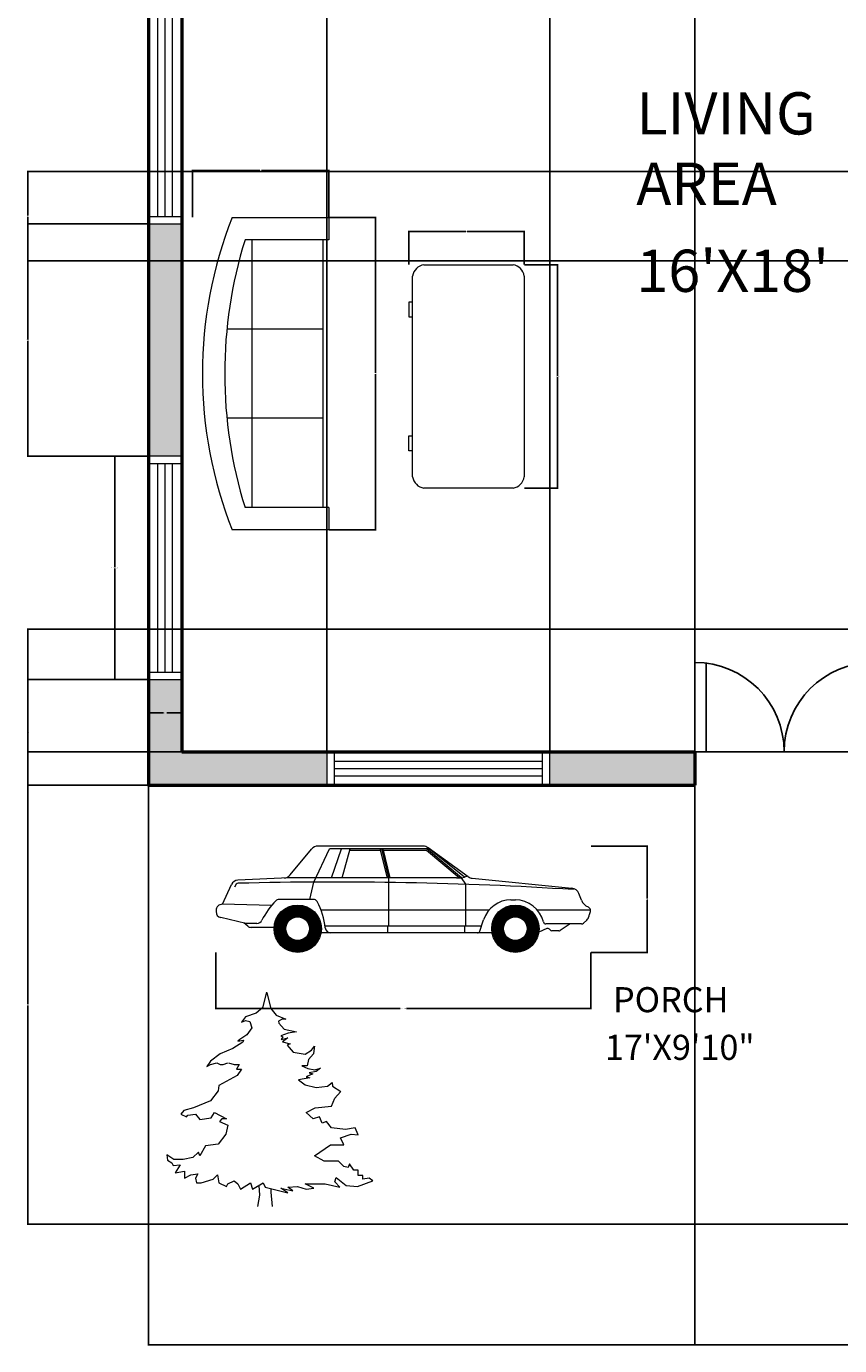
# Model space of a CAD drawing. Units: inches. Extents: x 96 to 522, y 502 to 1213.
# Tile 1 of 5: x 96 to 315, y 502 to 856. Entities that reach past the tile are written whole.
import ezdxf

# ---------------------------------------------------------------- set-up
doc = ezdxf.new("R2010")
doc.units = ezdxf.units.IN
doc.layers.get('Defpoints').update_dxf_attribs({"color": 90})
for name, color, linetype, lineweight in [('A-ANNO-DIMS', 2, 'Continuous', 18), ('A-AREA-IDEN', 7, 'Continuous', 25), ('A-DOOR', 3, 'Continuous', 25), ('A-FLOR', 7, 'Continuous', 25), ('A-FURN', 8, 'Continuous', 18), ('A-GLAZ', 4, 'Continuous', 18), ('A-SITE-VEHC', 8, 'Continuous', 13), ('A-WALL', 7, 'Continuous', 50), ('L-PLNT', 90, 'Continuous', 13)]:
    doc.layers.add(name, color=color, linetype=linetype, lineweight=lineweight)
doc.layers.add('A-WALL-PATT', color=252, linetype='Continuous', lineweight=13, true_color=0x939598)
doc.styles.get("Standard").update_dxf_attribs({"font": 'arial.ttf'})
doc.dimstyles.get("Standard").update_dxf_attribs({"dimtxt": 0.18, "dimasz": 0.18, "dimexe": 0.18, "dimexo": 0.0625, "dimgap": 0.09, "dimtad": 0, "dimtih": 1, "dimtoh": 1, "dimdec": 4, "dimzin": 0, "dimdsep": 46, "dimtxsty": 'Standard', "dimcen": 0.09, "dimadec": 0, "dimazin": 0, "dimtfac": 1, "dimtdec": 4, "dimtofl": 0, "dimtmove": 0, "dimatfit": 3, "dimfxl": 1, "dimtolj": 1, "dimtzin": 0, "dimarcsym": 0})

# ---------------------------------------------------------------- blocks, each defined once
blk = doc.blocks.new('Sofa - Roundback 7 ft.')
for p, q in [((-12.00002, -32.4421), (-12.00003, -6.5971)), ((11.99997, -32.4421), (11.99998, -6.5971)), ((-36.000027, -34), (-36.000027, -11.4696)), ((-35.999844, -13.3819), (35.9998, -13.3819)), ((35.99998, -34), (35.99998, -11.4696)), ((-36.000027, -32.4421), (35.99998, -32.4421))]:
    blk.add_line(p, q)
for points in [[(-36.000027, -34), (-42.000027, -34), (-42.000027, -8)], [(41.99998, -8), (41.99998, -34), (35.99998, -34)]]:
    blk.add_lwpolyline(points)
for centre, radius, start, end in [((0, -114.25), 114.25, 68.43141, 111.5686), ((-0.00001, -127.1968), 121.1968, 72.72033, 107.2797)]:
    blk.add_arc(centre, radius, start, end)
blk = doc.blocks.new('Desk - 30 x 60 in.')
for p, q in [((-26.999995, 0), (26.999995, 0)), ((-29.999995, -27), (-29.999995, -3)), ((29.999995, -3), (29.999995, -27)), ((26.999995, -30), (-26.999995, -30)), ((-20.000005, -30), (-20.000005, -31)), ((-20.000005, -31), (-16.000005, -31)), ((-16.000005, -31), (-16.000005, -30)), ((15.999995, -31), (15.999995, -30)), ((19.999995, -31), (15.999995, -31)), ((19.999995, -30), (19.999995, -31))]:
    blk.add_line(p, q)
for centre, start, end in [((-26.499995, -3.5), 98.1301, 171.8699), ((26.499995, -3.5), 8.130102, 81.8699), ((-26.499995, -26.5), 188.1301, 261.8699), ((26.499995, -26.5), 278.1301, 351.8699)]:
    blk.add_arc(centre, 3.535534, start, end)
blk = doc.blocks.new('Car - sedan  side')
for p, q in [((-77.81, 49.34), (-126.58, 49.34)), ((-139.53, 35.99), (-129.64, 47.91)), ((-128.57, 32.64), (-121.22, 48.02)), ((-74.7, 48.02), (-121.22, 48.02)), ((-120.32, 34.67), (-115.67, 48.02)), ((-115.4, 34.67), (-111.74, 48.02)), ((-97.55, 47.3), (-111.94, 47.3)), ((-94.41, 34.67), (-97.73, 48.02)), ((-93.72, 34.67), (-97.04, 48.02)), ((-93.03, 34.67), (-96.34, 48.02)), ((-76.26, 47.3), (-96.16, 47.3)), ((-61.08, 34.66), (-76.26, 47.3)), ((-60.02, 34.65), (-76.07, 48.02)), ((-56.87, 35.13), (-75.48, 48.59)), ((-58.54, 34.93), (-74.99, 48.02)), ((-170.93, 22.32), (-166.81, 31.56)), ((-164.57, 31.6), (-165.48, 30.35)), ((-140.23, 34.67), (-163.88, 33.56)), ((-62.28, 34.67), (-140.23, 34.67)), ((-130.39, 24.63), (-128.57, 32.64)), ((-93.72, 19.62), (-93.72, 34.67)), ((-62.28, 34.67), (-60.02, 34.65)), ((-60.02, 34.65), (-58.54, 34.93)), ((-57.97, 31.61), (-60.02, 34.65)), ((-57.21, 35.38), (-58.54, 34.93)), ((-57.97, 19.62), (-57.97, 31.61)), ((-54.93, 34.4), (-8.75, 29.8)), ((-128.78, 24.63), (-144.79, 24.63)), ((-4.21, 24.18), (-5.42, 27.27)), ((-174, 19.51), (-174, 18.91)), ((-148.26, 21.7), (-171.11, 22.33)), ((-47.2, 19.62), (-125.23, 19.62)), ((-93.72, 12.14), (-93.72, 19.62)), ((-57.97, 12.14), (-57.97, 19.62)), ((-36.97, 24.38), (-34.94, 24.38)), ((0, 19.62), (-24.7, 19.62)), ((-160.12, 13.48), (-171.81, 16.16)), ((-159.22, 12.14), (-161.08, 13.7)), ((-155.01, 13.48), (-160.12, 13.48)), ((-51.4, 9.89), (-49.69, 15.14)), ((-4.23, 13.19), (-20.72, 13.19)), ((-9.5, 13.19), (-14.1, 10.2)), ((-3.22, 13.59), (-1.77, 14.97)), ((-147.03, 11.6), (-157.73, 11.6)), ((-120.62, 9.03), (-125.23, 9.03)), ((-50.67, 12.14), (-123.32, 12.14)), ((-45.76, 9.03), (-120.62, 9.03)), ((-94.21, 9.03), (-94.21, 12.14)), ((-58.39, 9.03), (-58.39, 12.14)), ((-20.36, 11.06), (-24.06, 9.44)), ((-18.83, 10.42), (-19.11, 10.76)), ((-14.68, 10.03), (-18.01, 10.03))]:
    blk.add_line(p, q)
at = {"const_width": 5.49}
for points in [[(-127.8, 11, -1), (-144.3, 11, -1)], [(-26.69, 11, -1), (-43.19, 11, -1)]]:
    blk.add_lwpolyline(points, format="xyb", close=True, dxfattribs=at)
for centre, radius in [((-136.05, 11), 11), ((-34.94, 11), 11), ((-136.05, 11), 5.51), ((-34.94, 11), 5.51)]:
    blk.add_circle(centre, radius)
for centre, radius, start, end in [((-126.58, 45.38), 3.97, 90, 140.30288), ((-77.81, 45.38), 3.97, 54.13504, 90), ((-163.72, 30.18), 3.38, 92.68266, 155.97362), ((-163.62, 30.91), 1.17, 91.49105, 143.95527), ((-118.51, -1702.12), 1734.79, 86.34698, 91.49105), ((-142.58, 38.53), 3.97, 272.68265, 320.30288), ((-54.54, 38.35), 3.97, 234.13503, 264.31231), ((-144.79, 22.64), 1.98, 90, 136.3964), ((-128.78, 22.64), 1.98, 28.1371, 90), ((-9.15, 25.82), 4, 21.31069, 84.3123), ((-171.18, 19.51), 2.82, 88.41927, 180), ((-171.18, 18.91), 2.82, 180, 257.09053), ((-118.09, -2.78), 38.85, 136.3964, 152.90974), ((-157.14, 7.48), 34.14, 6.51354, 28.1371), ((-36.97, 11), 13.38, 90, 161.97316), ((-34.94, 11), 13.38, 13.58642, 90), ((0.9, 26.18), 5.49, 201.3107, 247.70484), ((-1.92, 19.3), 1.94, 325.37436, 67.70485), ((-155.01, 16.1), 2.62, 270, 332.90974), ((-20.72, 14.43), 1.24, 193.58641, 270), ((-4.23, 14.65), 1.46, 270, 313.71735), ((-3.82, 17.12), 2.96, 313.71735, 352.38387), ((2.46, 16.28), 3.37, 145.37437, 172.38386), ((-157.73, 13.93), 2.32, 230.12913, 270), ((-120.62, 11.65), 2.62, 186.51353, 270), ((-52.58, 10.27), 1.24, 270, 341.97316), ((-19.93, 10.09), 1.06, 39.30103, 113.71592), ((-18.01, 11.09), 1.06, 219.30104, 270), ((-14.68, 11.09), 1.06, 270, 303.04697)]:
    blk.add_arc(centre, radius, start, end)
blk = doc.blocks.new('WIN-60IN')
for p, q in [((60, 9), (0, 9)), ((0, 9), (0, 0)), ((2, 9), (2, 0)), ((58, 0), (58, 9)), ((60, 0), (60, 9)), ((2, 6.5), (58, 6.5)), ((2, 4.5), (58, 4.5)), ((0, 0), (60, 0)), ((2, 2.5), (58, 2.5))]:
    blk.add_line(p, q)
blk = doc.blocks.new('DOOR-DBL-48IN')
for p, q in [((0, 24), (0, 0)), ((3, 24), (3, 0)), ((45, 24), (45, 0)), ((48, 24), (48, 0)), ((0, 0), (3, 0)), ((48, 0), (45, 0))]:
    blk.add_line(p, q)
for centre, start, end in [((0, 0), 0, 90), ((48, 0), 90, 180)]:
    blk.add_arc(centre, 24, start, end)
blk = doc.blocks.new('*D17')
at = {"layer": 'A-ANNO-DIMS', "color": 0, "lineweight": -2, "transparency": 16777216}
for p, q in [((129.15, 740.69), (120.03, 740.69)), ((120.21, 740.51), (120.21, 710.88)), ((120.21, 680.87), (120.21, 710.51)), ((129.15, 680.69), (120.03, 680.69))]:
    blk.add_line(p, q, dxfattribs=at)
at = {"layer": 'A-ANNO-DIMS', "color": 0, "transparency": 16777216}
for points in [[(120.18, 740.51), (120.24, 740.51), (120.21, 740.69)], [(120.18, 680.87), (120.24, 680.87), (120.21, 680.69)]]:
    blk.add_solid(points, dxfattribs=at)
at = {"layer": 'Defpoints', "color": 0, "transparency": 16777216}
for p in [(120.21, 740.69), (129.21, 740.69), (129.21, 680.69)]:
    blk.add_point(p, dxfattribs=at)
at = {"layer": 'A-ANNO-DIMS', "color": 0, "transparency": 16777216, "insert": (120.21, 710.69), "char_height": 0.18, "attachment_point": 5}
blk.add_mtext('\\A1;WINDOW 60 TYP.', dxfattribs=at)
blk = doc.blocks.new('*D18')
at = {"layer": 'A-ANNO-DIMS', "color": 0, "lineweight": -2, "transparency": 16777216}
for p, q in [((129.21, 680.63), (129.21, 671.51)), ((138.21, 680.63), (138.21, 671.51)), ((129.39, 671.69), (133.25, 671.69)), ((138.03, 671.69), (134.17, 671.69))]:
    blk.add_line(p, q, dxfattribs=at)
at = {"layer": 'A-ANNO-DIMS', "color": 0, "transparency": 16777216}
for points in [[(129.39, 671.72), (129.39, 671.66), (129.21, 671.69)], [(138.03, 671.72), (138.03, 671.66), (138.21, 671.69)]]:
    blk.add_solid(points, dxfattribs=at)
at = {"layer": 'Defpoints', "color": 0, "transparency": 16777216}
for p in [(129.21, 680.69), (138.21, 680.69), (129.21, 671.69)]:
    blk.add_point(p, dxfattribs=at)
at = {"layer": 'A-ANNO-DIMS', "color": 0, "transparency": 16777216, "insert": (133.71, 671.69), "char_height": 0.18, "attachment_point": 5}
blk.add_mtext('\\A1;9 TYP.', dxfattribs=at)
blk = doc.blocks.new('*D35')
at = {"layer": 'A-ANNO-DIMS', "color": 0, "lineweight": -2, "transparency": 16777216}
for p, q in [((177.8, 804.9), (190.51, 804.9)), ((190.33, 804.72), (190.33, 763.09)), ((190.33, 721.08), (190.33, 762.72)), ((177.8, 720.9), (190.51, 720.9))]:
    blk.add_line(p, q, dxfattribs=at)
at = {"layer": 'A-ANNO-DIMS', "color": 0, "transparency": 16777216}
for points in [[(190.3, 804.72), (190.36, 804.72), (190.33, 804.9)], [(190.3, 721.08), (190.36, 721.08), (190.33, 720.9)]]:
    blk.add_solid(points, dxfattribs=at)
at = {"layer": 'Defpoints', "color": 0, "transparency": 16777216}
for p in [(177.73, 804.9), (190.33, 804.9), (177.73, 720.9)]:
    blk.add_point(p, dxfattribs=at)
at = {"layer": 'A-ANNO-DIMS', "color": 0, "transparency": 16777216, "insert": (190.33, 762.9), "char_height": 0.18, "attachment_point": 5}
blk.add_mtext('\\A1;SOFA 84', dxfattribs=at)
blk = doc.blocks.new('*D36')
at = {"layer": 'A-ANNO-DIMS', "color": 0, "lineweight": -2, "transparency": 16777216}
for p, q in [((141.07, 804.96), (141.07, 817.68)), ((141.25, 817.5), (159.18, 817.5)), ((177.55, 817.5), (159.62, 817.5)), ((177.73, 804.96), (177.73, 817.68))]:
    blk.add_line(p, q, dxfattribs=at)
at = {"layer": 'A-ANNO-DIMS', "color": 0, "transparency": 16777216}
for points in [[(141.25, 817.53), (141.25, 817.47), (141.07, 817.5)], [(177.55, 817.53), (177.55, 817.47), (177.73, 817.5)]]:
    blk.add_solid(points, dxfattribs=at)
at = {"layer": 'Defpoints', "color": 0, "transparency": 16777216}
for p in [(141.07, 817.5), (141.07, 804.9), (177.73, 804.9)]:
    blk.add_point(p, dxfattribs=at)
at = {"layer": 'A-ANNO-DIMS', "color": 0, "transparency": 16777216, "insert": (159.4, 817.5), "char_height": 0.18, "attachment_point": 5}
blk.add_mtext('\\A1;37', dxfattribs=at)
blk = doc.blocks.new('*D37')
at = {"layer": 'A-ANNO-DIMS', "color": 0, "lineweight": -2, "transparency": 16777216}
for p, q in [((230.35, 792.15), (239.47, 792.15)), ((239.29, 791.97), (239.29, 762.33)), ((239.29, 732.33), (239.29, 761.97)), ((230.35, 732.15), (239.47, 732.15))]:
    blk.add_line(p, q, dxfattribs=at)
at = {"layer": 'A-ANNO-DIMS', "color": 0, "transparency": 16777216}
for points in [[(239.26, 791.97), (239.32, 791.97), (239.29, 792.15)], [(239.26, 732.33), (239.32, 732.33), (239.29, 732.15)]]:
    blk.add_solid(points, dxfattribs=at)
at = {"layer": 'Defpoints', "color": 0, "transparency": 16777216}
for p in [(230.29, 792.15), (230.29, 732.15), (239.29, 732.15)]:
    blk.add_point(p, dxfattribs=at)
at = {"layer": 'A-ANNO-DIMS', "color": 0, "transparency": 16777216, "insert": (239.29, 762.15), "char_height": 0.18, "attachment_point": 5}
blk.add_mtext('\\A1;DESK 60', dxfattribs=at)
blk = doc.blocks.new('*D38')
at = {"layer": 'A-ANNO-DIMS', "color": 0, "lineweight": -2, "transparency": 16777216}
for p, q in [((199.29, 792.21), (199.29, 801.33)), ((199.47, 801.15), (214.58, 801.15)), ((230.11, 801.15), (214.99, 801.15)), ((230.29, 792.21), (230.29, 801.33))]:
    blk.add_line(p, q, dxfattribs=at)
at = {"layer": 'A-ANNO-DIMS', "color": 0, "transparency": 16777216}
for points in [[(199.47, 801.18), (199.47, 801.12), (199.29, 801.15)], [(230.11, 801.18), (230.11, 801.12), (230.29, 801.15)]]:
    blk.add_solid(points, dxfattribs=at)
at = {"layer": 'Defpoints', "color": 0, "transparency": 16777216}
for p in [(230.29, 801.15), (199.29, 792.15), (230.29, 792.15)]:
    blk.add_point(p, dxfattribs=at)
at = {"layer": 'A-ANNO-DIMS', "color": 0, "transparency": 16777216, "insert": (214.79, 801.15), "char_height": 0.18, "attachment_point": 5}
blk.add_mtext('\\A1;31', dxfattribs=at)
blk = doc.blocks.new('*D45')
at = {"layer": 'A-ANNO-DIMS', "color": 0, "lineweight": -2, "transparency": 16777216}
for p, q in [((147.39, 607.26), (147.39, 592.02)), ((248.21, 607.26), (248.21, 592.02)), ((147.57, 592.2), (196.95, 592.2)), ((248.03, 592.2), (198.65, 592.2))]:
    blk.add_line(p, q, dxfattribs=at)
at = {"layer": 'A-ANNO-DIMS', "color": 0, "transparency": 16777216}
for points in [[(147.57, 592.23), (147.57, 592.17), (147.39, 592.2)], [(248.03, 592.23), (248.03, 592.17), (248.21, 592.2)]]:
    blk.add_solid(points, dxfattribs=at)
at = {"layer": 'Defpoints', "color": 0, "transparency": 16777216}
for p in [(147.39, 607.32), (248.21, 607.32), (248.21, 592.2)]:
    blk.add_point(p, dxfattribs=at)
at = {"layer": 'A-ANNO-DIMS', "color": 0, "transparency": 16777216, "insert": (197.8, 592.2), "char_height": 0.18, "attachment_point": 5}
blk.add_mtext('\\A1;VEHICLE 101', dxfattribs=at)
blk = doc.blocks.new('*D46')
at = {"layer": 'A-ANNO-DIMS', "color": 0, "lineweight": -2, "transparency": 16777216}
for p, q in [((248.28, 635.9), (263.52, 635.9)), ((263.34, 635.72), (263.34, 621.79)), ((263.34, 607.5), (263.34, 621.43)), ((248.28, 607.32), (263.52, 607.32))]:
    blk.add_line(p, q, dxfattribs=at)
at = {"layer": 'A-ANNO-DIMS', "color": 0, "transparency": 16777216}
for points in [[(263.31, 635.72), (263.37, 635.72), (263.34, 635.9)], [(263.31, 607.5), (263.37, 607.5), (263.34, 607.32)]]:
    blk.add_solid(points, dxfattribs=at)
at = {"layer": 'Defpoints', "color": 0, "transparency": 16777216}
for p in [(248.21, 635.9), (263.34, 635.9), (248.21, 607.32)]:
    blk.add_point(p, dxfattribs=at)
at = {"layer": 'A-ANNO-DIMS', "color": 0, "transparency": 16777216, "insert": (263.34, 621.61), "char_height": 0.18, "attachment_point": 5}
blk.add_mtext('\\A1;29', dxfattribs=at)
blk = doc.blocks.new('*D47')
at = {"layer": 'A-ANNO-DIMS', "color": 0, "lineweight": -2, "transparency": 16777216}
for p, q in [((129.21, 534.19), (129.21, 501.62)), ((489.21, 534.19), (489.21, 501.62)), ((129.39, 501.8), (308.92, 501.8)), ((489.03, 501.8), (309.5, 501.8))]:
    blk.add_line(p, q, dxfattribs=at)
at = {"layer": 'A-ANNO-DIMS', "color": 0, "transparency": 16777216}
for points in [[(129.39, 501.83), (129.39, 501.77), (129.21, 501.8)], [(489.03, 501.83), (489.03, 501.77), (489.21, 501.8)]]:
    blk.add_solid(points, dxfattribs=at)
at = {"layer": 'Defpoints', "color": 0, "transparency": 16777216}
for p in [(129.21, 534.25), (489.21, 534.25), (489.21, 501.8)]:
    blk.add_point(p, dxfattribs=at)
at = {"layer": 'A-ANNO-DIMS', "color": 0, "transparency": 16777216, "insert": (309.21, 501.8), "char_height": 0.18, "attachment_point": 5}
blk.add_mtext('\\A1;360', dxfattribs=at)
blk = doc.blocks.new('*D49')
at = {"layer": 'A-ANNO-DIMS', "color": 0, "lineweight": -2, "transparency": 16777216}
for p, q in [((129.15, 652.25), (96.58, 652.25)), ((96.76, 652.07), (96.76, 593.43)), ((96.76, 534.43), (96.76, 593.07)), ((129.15, 534.25), (96.58, 534.25))]:
    blk.add_line(p, q, dxfattribs=at)
at = {"layer": 'A-ANNO-DIMS', "color": 0, "transparency": 16777216}
for points in [[(96.73, 652.07), (96.79, 652.07), (96.76, 652.25)], [(96.73, 534.43), (96.79, 534.43), (96.76, 534.25)]]:
    blk.add_solid(points, dxfattribs=at)
at = {"layer": 'Defpoints', "color": 0, "transparency": 16777216}
for p in [(96.76, 652.25), (129.21, 652.25), (129.21, 534.25)]:
    blk.add_point(p, dxfattribs=at)
at = {"layer": 'A-ANNO-DIMS', "color": 0, "transparency": 16777216, "insert": (96.76, 593.25), "char_height": 0.18, "attachment_point": 5}
blk.add_mtext('\\A1;118', dxfattribs=at)
blk = doc.blocks.new('*D53')
at = {"layer": 'A-ANNO-DIMS', "color": 0, "lineweight": -2, "transparency": 16777216}
for p, q in [((138.21, 661.31), (138.21, 1212.88)), ((177.21, 661.31), (177.21, 1212.88)), ((138.39, 1212.7), (157.49, 1212.7)), ((177.03, 1212.7), (157.93, 1212.7))]:
    blk.add_line(p, q, dxfattribs=at)
at = {"layer": 'A-ANNO-DIMS', "color": 0, "transparency": 16777216}
for points in [[(138.39, 1212.73), (138.39, 1212.67), (138.21, 1212.7)], [(177.03, 1212.73), (177.03, 1212.67), (177.21, 1212.7)]]:
    blk.add_solid(points, dxfattribs=at)
at = {"layer": 'Defpoints', "color": 0, "transparency": 16777216}
for p in [(177.21, 1212.7), (138.21, 661.25), (177.21, 661.25)]:
    blk.add_point(p, dxfattribs=at)
at = {"layer": 'A-ANNO-DIMS', "color": 0, "transparency": 16777216, "insert": (157.71, 1212.7), "char_height": 0.18, "attachment_point": 5}
blk.add_mtext('\\A1;39', dxfattribs=at)
blk = doc.blocks.new('*D54')
at = {"layer": 'A-ANNO-DIMS', "color": 0, "lineweight": -2, "transparency": 16777216}
for p, q in [((237.21, 661.31), (237.21, 1212.88)), ((276.21, 661.31), (276.21, 1212.88)), ((237.39, 1212.7), (256.49, 1212.7)), ((276.03, 1212.7), (256.93, 1212.7))]:
    blk.add_line(p, q, dxfattribs=at)
at = {"layer": 'A-ANNO-DIMS', "color": 0, "transparency": 16777216}
for points in [[(237.39, 1212.73), (237.39, 1212.67), (237.21, 1212.7)], [(276.03, 1212.73), (276.03, 1212.67), (276.21, 1212.7)]]:
    blk.add_solid(points, dxfattribs=at)
at = {"layer": 'Defpoints', "color": 0, "transparency": 16777216}
for p in [(276.21, 1212.7), (237.21, 661.25), (276.21, 661.25)]:
    blk.add_point(p, dxfattribs=at)
at = {"layer": 'A-ANNO-DIMS', "color": 0, "transparency": 16777216, "insert": (256.71, 1212.7), "char_height": 0.18, "attachment_point": 5}
blk.add_mtext('\\A1;39', dxfattribs=at)
blk = doc.blocks.new('*D56')
at = {"layer": 'A-ANNO-DIMS', "color": 0, "lineweight": -2, "transparency": 16777216}
for p, q in [((129.15, 680.69), (96.58, 680.69)), ((96.76, 680.51), (96.76, 666.65)), ((96.76, 652.43), (96.76, 666.29)), ((129.15, 652.25), (96.58, 652.25))]:
    blk.add_line(p, q, dxfattribs=at)
at = {"layer": 'A-ANNO-DIMS', "color": 0, "transparency": 16777216}
for points in [[(96.73, 680.51), (96.79, 680.51), (96.76, 680.69)], [(96.73, 652.43), (96.79, 652.43), (96.76, 652.25)]]:
    blk.add_solid(points, dxfattribs=at)
at = {"layer": 'Defpoints', "color": 0, "transparency": 16777216}
for p in [(96.76, 680.69), (129.21, 680.69), (129.21, 652.25)]:
    blk.add_point(p, dxfattribs=at)
at = {"layer": 'A-ANNO-DIMS', "color": 0, "transparency": 16777216, "insert": (96.76, 666.47), "char_height": 0.18, "attachment_point": 5}
blk.add_mtext('\\A1;28.444', dxfattribs=at)
blk = doc.blocks.new('*D57')
at = {"layer": 'A-ANNO-DIMS', "color": 0, "lineweight": -2, "transparency": 16777216}
for p, q in [((129.15, 803.14), (96.58, 803.14)), ((96.76, 802.96), (96.76, 772.1)), ((96.76, 740.87), (96.76, 771.74)), ((129.15, 740.69), (96.58, 740.69))]:
    blk.add_line(p, q, dxfattribs=at)
at = {"layer": 'A-ANNO-DIMS', "color": 0, "transparency": 16777216}
for points in [[(96.73, 802.96), (96.79, 802.96), (96.76, 803.14)], [(96.73, 740.87), (96.79, 740.87), (96.76, 740.69)]]:
    blk.add_solid(points, dxfattribs=at)
at = {"layer": 'Defpoints', "color": 0, "transparency": 16777216}
for p in [(96.76, 803.14), (129.21, 803.14), (129.21, 740.69)]:
    blk.add_point(p, dxfattribs=at)
at = {"layer": 'A-ANNO-DIMS', "color": 0, "transparency": 16777216, "insert": (96.76, 771.92), "char_height": 0.18, "attachment_point": 5}
blk.add_mtext('\\A1;62.44', dxfattribs=at)
blk = doc.blocks.new('*D60')
at = {"layer": 'A-ANNO-DIMS', "color": 0, "lineweight": -2, "transparency": 16777216}
for p, q in [((480.15, 694.25), (96.58, 694.25)), ((96.76, 694.07), (96.76, 677.93)), ((96.76, 661.43), (96.76, 677.57)), ((480.15, 661.25), (96.58, 661.25))]:
    blk.add_line(p, q, dxfattribs=at)
at = {"layer": 'A-ANNO-DIMS', "color": 0, "transparency": 16777216}
for points in [[(96.73, 694.07), (96.79, 694.07), (96.76, 694.25)], [(96.73, 661.43), (96.79, 661.43), (96.76, 661.25)]]:
    blk.add_solid(points, dxfattribs=at)
at = {"layer": 'Defpoints', "color": 0, "transparency": 16777216}
for p in [(96.76, 694.25), (480.21, 694.25), (480.21, 661.25)]:
    blk.add_point(p, dxfattribs=at)
at = {"layer": 'A-ANNO-DIMS', "color": 0, "transparency": 16777216, "insert": (96.76, 677.75), "char_height": 0.18, "attachment_point": 5}
blk.add_mtext('\\A1;33', dxfattribs=at)
blk = doc.blocks.new('*D61')
at = {"layer": 'A-ANNO-DIMS', "color": 0, "lineweight": -2, "transparency": 16777216}
for p, q in [((480.15, 817.25), (96.58, 817.25)), ((96.76, 817.07), (96.76, 805.43)), ((96.76, 793.43), (96.76, 805.07)), ((480.15, 793.25), (96.58, 793.25))]:
    blk.add_line(p, q, dxfattribs=at)
at = {"layer": 'A-ANNO-DIMS', "color": 0, "transparency": 16777216}
for points in [[(96.73, 817.07), (96.79, 817.07), (96.76, 817.25)], [(96.73, 793.43), (96.79, 793.43), (96.76, 793.25)]]:
    blk.add_solid(points, dxfattribs=at)
at = {"layer": 'Defpoints', "color": 0, "transparency": 16777216}
for p in [(96.76, 817.25), (480.21, 817.25), (480.21, 793.25)]:
    blk.add_point(p, dxfattribs=at)
at = {"layer": 'A-ANNO-DIMS', "color": 0, "transparency": 16777216, "insert": (96.76, 805.25), "char_height": 0.18, "attachment_point": 5}
blk.add_mtext('\\A1;24', dxfattribs=at)
blk = doc.blocks.new('*D66')
at = {"layer": 'A-ANNO-DIMS', "color": 0, "lineweight": -2, "transparency": 16777216}
for p, q in [((330.21, 1033.19), (330.21, 501.62)), ((276.21, 997.19), (276.21, 501.62)), ((276.39, 501.8), (302.99, 501.8)), ((330.03, 501.8), (303.43, 501.8))]:
    blk.add_line(p, q, dxfattribs=at)
at = {"layer": 'A-ANNO-DIMS', "color": 0, "transparency": 16777216}
for points in [[(276.39, 501.83), (276.39, 501.77), (276.21, 501.8)], [(330.03, 501.83), (330.03, 501.77), (330.21, 501.8)]]:
    blk.add_solid(points, dxfattribs=at)
at = {"layer": 'Defpoints', "color": 0, "transparency": 16777216}
for p in [(330.21, 1033.25), (276.21, 997.25), (330.21, 501.8)]:
    blk.add_point(p, dxfattribs=at)
at = {"layer": 'A-ANNO-DIMS', "color": 0, "transparency": 16777216, "insert": (303.21, 501.8), "char_height": 0.18, "attachment_point": 5}
blk.add_mtext('\\A1;54', dxfattribs=at)

msp = doc.modelspace()

# ---------------------------------------------------------------- hatches: boundary and pattern name
at = {"layer": 'A-WALL-PATT'}
h = msp.add_hatch(color=256, dxfattribs=at)
h.dxf.hatch_style = 1
h.paths.add_polyline_path([(174.2111, 1156.2511), (129.2111, 1156.2511), (129.2111, 1105.2511), (138.2111, 1105.2511), (138.2111, 1147.2511), (174.2111, 1147.2511)])
h.paths.add_polyline_path([(287.2111, 1156.2511), (234.2111, 1156.2511), (234.2111, 1147.2511), (270.2111, 1147.2511), (270.2111, 1003.2511), (267.2111, 1003.2511), (267.2111, 997.2511), (276.2111, 997.2511), (276.2111, 1147.2511), (287.2111, 1147.2511)])
h.paths.add_polyline_path([(342.2111, 1156.2511), (335.2111, 1156.2511), (335.2111, 1147.2511), (338.2111, 1147.2511), (338.2111, 1081.2511), (342.2111, 1081.2511), (342.2111, 1147.2511)])
h.paths.add_polyline_path([(489.2111, 1156.2511), (402.2111, 1156.2511), (402.2111, 1147.2511), (402.2111, 1141.2511), (408.2111, 1141.2511), (408.2111, 1147.2511), (480.2111, 1147.2511), (480.2111, 1123.2511), (489.2111, 1123.2511)])
h.paths.add_polyline_path([(489.2111, 1111.2511), (480.2111, 1111.2511), (480.2111, 1087.2511), (408.2111, 1087.2511), (408.2111, 1111.2511), (402.2111, 1111.2511), (402.2111, 1066.2511), (408.2111, 1066.2511), (408.2111, 1081.2511), (480.2111, 1081.2511), (480.2111, 1063.2511), (489.2111, 1063.2511)])
h.paths.add_polyline_path([(489.2111, 1051.2511), (480.2111, 1051.2511), (480.2111, 1033.2511), (408.2111, 1033.2511), (408.2111, 1036.2511), (402.2111, 1036.2511), (402.2111, 1033.2511), (338.2111, 1033.2511), (330.2111, 1033.2511), (330.2111, 923.2511), (336.2111, 923.2511), (336.2111, 1027.2511), (338.2111, 1027.2511), (402.2111, 1027.2511), (480.2111, 1027.2511), (480.2111, 973.2511), (489.2111, 973.2511)])
h.paths.add_polyline_path([(489.2111, 913.2511), (480.2111, 913.2511), (480.2111, 859.2511), (429.2111, 859.2511), (429.2111, 853.2511), (480.2111, 853.2511), (480.2111, 829.2511), (489.2111, 829.2511)])
h.paths.add_polyline_path([(489.2111, 817.2511), (480.2111, 817.2511), (480.2111, 793.2511), (402.2111, 793.2511), (396.2111, 793.2511), (396.2111, 853.2511), (399.2111, 853.2511), (399.2111, 859.2511), (338.2111, 859.2511), (336.2111, 859.2511), (336.2111, 877.2511), (336.2111, 883.2511), (336.2111, 887.2511), (330.2111, 887.2511), (330.2111, 883.2511), (326.2111, 883.2511), (326.2111, 877.2511), (330.2111, 877.2511), (330.2111, 853.2511), (338.2111, 853.2511), (390.2111, 853.2511), (390.2111, 793.2511), (387.2111, 793.2511), (387.2111, 787.2511), (402.2111, 787.2511), (480.2111, 787.2511), (480.2111, 754.2511), (489.2111, 754.2511)])
h.paths.add_polyline_path([(489.2111, 694.2511), (480.2111, 694.2511), (480.2111, 661.2511), (432.2111, 661.2511), (432.2111, 652.2511), (480.2111, 652.2511), (480.2111, 543.2511), (333.2111, 543.2511), (333.2111, 534.2511), (489.2111, 534.2511), (489.2111, 652.2511)])
h.paths.add_polyline_path([(372.2111, 661.2511), (336.2111, 661.2511), (336.2111, 787.2511), (338.2111, 787.2511), (351.2111, 787.2511), (351.2111, 793.2511), (338.2111, 793.2511), (330.2111, 793.2511), (330.2111, 661.2511), (324.2111, 661.2511), (324.2111, 652.2511), (372.2111, 652.2511)])
h.paths.add_polyline_path([(138.2111, 680.6946), (129.2111, 680.6946), (129.2111, 652.2511), (177.2111, 652.2511), (177.2111, 661.2511), (138.2111, 661.2511)])
h.paths.add_polyline_path([(276.2111, 661.2511), (237.2111, 661.2511), (237.2111, 652.2511), (276.2111, 652.2511)])
h.paths.add_polyline_path([(138.2111, 803.1393), (129.2111, 803.1393), (129.2111, 740.6946), (138.2111, 740.6946)])
h.paths.add_polyline_path([(138.2111, 907.2511), (129.2111, 907.2511), (129.2111, 863.1393), (138.2111, 863.1393), (138.2111, 877.2511), (276.2111, 877.2511), (276.2111, 883.2511), (204.2111, 883.2511), (204.2111, 886.2511), (198.2111, 886.2511), (198.2111, 883.2511), (138.2111, 883.2511)])
h.paths.add_polyline_path([(138.2111, 943.2511), (198.2111, 943.2511), (198.2111, 916.2511), (204.2111, 916.2511), (204.2111, 949.2511), (138.2111, 949.2511), (138.2111, 997.2511), (231.2111, 997.2511), (231.2111, 1003.2511), (138.2111, 1003.2511), (138.2111, 1045.2511), (129.2111, 1045.2511), (129.2111, 919.2511), (138.2111, 919.2511)])

# ---------------------------------------------------------------- linework, layer by layer
at = {"layer": 'A-FLOR'}
for p, q in [((129.2111, 652.2511), (129.2111, 534.2511)), ((129.2111, 534.2511), (333.2111, 534.2511))]:
    msp.add_line(p, q, dxfattribs=at)
at = {"layer": 'A-WALL'}
for p, q in [((138.2111, 877.2511), (138.2111, 661.2511)), ((138.2111, 661.2511), (276.2111, 661.2511)), ((276.2111, 661.2511), (276.2111, 652.2511))]:
    msp.add_line(p, q, dxfattribs=at)
msp.add_lwpolyline([(287.2111, 1156.2511), (129.2111, 1156.2511), (129.2111, 652.2511), (276.2111, 652.2511)], dxfattribs=at)
at = {"layer": 'L-PLNT'}
for p, q in [((160.978, 596.5966), (159.887, 592.4232)), ((161.0351, 596.4428), (162.1216, 592.2637)), ((159.887, 592.4232), (158.1853, 590.9688)), ((162.1216, 592.2637), (163.5424, 590.4419)), ((155.349, 589.9992), (154.2143, 588.5444)), ((154.2143, 588.5444), (155.349, 589.0292)), ((158.1853, 590.9688), (155.349, 589.9992)), ((155.349, 589.0292), (156.4833, 588.7868)), ((156.4833, 588.7868), (157.0506, 587.09)), ((163.5424, 590.4419), (166.1336, 589.3703)), ((165.2141, 589.3703), (164.2114, 588.8345)), ((164.2114, 588.8345), (164.2947, 588.2991)), ((166.1336, 589.3703), (165.2141, 589.3703)), ((155.7269, 585.1504), (153.8359, 583.9384)), ((157.0506, 587.09), (155.7269, 585.1504)), ((164.2947, 588.2991), (165.7155, 586.6918)), ((166.8021, 585.6202), (164.7961, 584.8699)), ((165.7155, 586.6918), (169.059, 585.9415)), ((169.059, 585.9415), (166.8021, 585.6202)), ((154.5922, 583.2112), (151.9448, 581.514)), ((153.8359, 583.9384), (153.2685, 583.4536)), ((153.2685, 583.4536), (154.7816, 583.696)), ((154.7816, 583.696), (154.5922, 583.2112)), ((164.7961, 584.8699), (165.3813, 584.6559)), ((165.3813, 584.6559), (164.9632, 583.9056)), ((164.9632, 583.9056), (166.7187, 584.3341)), ((166.7187, 584.3341), (165.2979, 583.263)), ((165.2979, 583.263), (167.3039, 582.7272)), ((167.3039, 582.7272), (166.5516, 582.4055)), ((166.5516, 582.4055), (168.1395, 580.4768)), ((173.0709, 581.0126), (173.9066, 582.0841)), ((173.9066, 582.0841), (173.8232, 581.5484)), ((145.8937, 578.1203), (144.9484, 576.6655)), ((148.5411, 580.0596), (145.8937, 578.1203)), ((151.9448, 581.514), (148.5411, 580.0596)), ((168.1395, 580.4768), (171.3992, 579.941)), ((171.3992, 579.941), (173.0709, 581.0126)), ((172.3186, 578.5481), (171.9006, 576.8335)), ((173.6561, 580.0482), (172.3186, 578.5481)), ((173.8232, 581.5484), (173.6561, 580.0482)), ((144.9484, 576.6655), (145.8937, 577.1503)), ((145.8937, 577.1503), (147.5958, 577.6351)), ((147.5958, 577.6351), (148.5411, 577.1503)), ((148.5411, 577.1503), (149.2975, 577.1503)), ((149.2975, 577.1503), (150.6212, 577.6351)), ((150.7195, 577.6578), (152.3232, 577.1503)), ((152.3232, 577.1503), (153.6469, 577.1503)), ((153.6469, 577.1503), (152.8906, 575.9383)), ((152.8906, 575.9383), (154.2143, 575.9383)), ((154.2143, 575.9383), (153.0796, 574.2415)), ((171.9006, 576.8335), (170.4798, 576.8335)), ((170.4798, 576.8335), (172.0681, 576.0836)), ((173.4052, 574.6907), (171.6501, 573.8332)), ((172.0681, 576.0836), (173.9903, 575.7623)), ((174.3246, 575.3333), (172.4858, 574.9048)), ((172.4858, 574.9048), (173.4052, 574.6907)), ((173.9903, 575.7623), (175.4949, 576.1909)), ((175.4949, 576.1909), (174.3246, 575.3333)), ((148.1632, 571.5747), (147.9738, 570.1203)), ((153.0796, 574.2415), (148.1632, 571.5747)), ((172.6529, 573.6191), (169.5604, 573.0834)), ((169.5604, 573.0834), (171.3992, 571.6905)), ((171.3992, 571.6905), (174.3246, 571.0474)), ((171.6501, 573.8332), (172.6529, 573.6191)), ((174.3246, 571.0474), (177.4171, 571.3687)), ((177.4171, 571.3687), (178.6708, 572.3331)), ((178.6708, 572.3331), (178.7546, 571.3687)), ((178.7546, 571.3687), (180.9277, 569.9759)), ((145.8937, 567.4535), (141.3557, 565.5143)), ((147.9738, 570.1203), (145.8937, 567.4535)), ((178.4187, 565.9991), (179.3644, 568.1807)), ((179.3644, 568.1807), (180.8771, 569.8779)), ((138.7083, 564.7867), (137.952, 563.8171)), ((141.3557, 565.5143), (138.7083, 564.7867)), ((146.0831, 562.8475), (147.0284, 564.3019)), ((147.0284, 564.3019), (150.2432, 562.6051)), ((171.6112, 564.3019), (174.0697, 565.5143)), ((173.5023, 562.6051), (171.6112, 564.3019)), ((174.0697, 565.5143), (178.4187, 565.9991)), ((137.952, 563.8171), (139.4647, 563.0899)), ((139.4647, 563.0899), (139.8426, 563.5747)), ((139.8426, 563.5747), (141.9231, 563.8171)), ((141.9231, 563.8171), (143.0574, 562.3627)), ((143.0574, 562.3627), (146.0831, 562.8475)), ((148.9195, 562.6051), (148.3521, 561.8779)), ((148.3521, 561.8779), (150.6212, 560.9079)), ((150.2432, 562.6051), (148.9195, 562.6051)), ((150.6212, 560.9079), (150.0542, 558.4839)), ((175.204, 563.0899), (173.5023, 562.6051)), ((175.9603, 561.3927), (175.204, 563.0899)), ((177.095, 561.8779), (175.9603, 561.3927)), ((178.4187, 560.1807), (177.095, 561.8779)), ((150.0542, 558.4839), (147.9738, 555.8171)), ((182.2008, 559.6959), (178.4187, 560.1807)), ((180.8771, 557.5143), (183.7135, 558.4839)), ((181.8224, 555.5747), (180.8771, 557.5143)), ((184.8482, 560.1807), (182.2008, 559.6959)), ((183.7135, 558.4839), (185.6045, 558.2415)), ((185.6045, 558.2415), (184.8482, 560.1807)), ((142.6794, 553.6355), (141.1663, 552.1807)), ((143.0574, 552.6655), (142.6794, 553.6355)), ((144.57, 555.3323), (143.0574, 552.6655)), ((147.9738, 555.8171), (144.57, 555.3323)), ((173.8803, 552.6655), (178.2297, 555.5747)), ((178.2297, 555.5747), (181.8224, 555.5747)), ((136.0609, 551.6959), (134.1699, 552.9079)), ((134.1699, 552.9079), (134.3589, 551.4535)), ((134.3589, 551.4535), (135.4936, 550.7263)), ((135.4936, 550.7263), (135.8716, 549.9991)), ((135.8716, 549.9991), (137.7626, 550.2415)), ((138.5189, 551.6959), (136.0609, 551.6959)), ((137.7626, 550.2415), (136.4389, 548.0595)), ((141.1663, 552.1807), (138.5189, 551.6959)), ((176.5276, 551.2111), (173.8803, 552.6655)), ((178.2297, 551.2111), (176.5276, 551.2111)), ((180.3097, 551.2111), (178.2297, 551.2111)), ((181.8224, 549.7567), (180.3097, 551.2111)), ((182.9571, 549.5143), (181.8224, 549.7567)), ((183.3355, 550.4839), (182.9571, 549.5143)), ((184.4698, 548.7867), (183.3355, 550.4839)), ((136.4389, 548.0595), (138.8973, 548.5443)), ((138.8973, 548.5443), (138.8973, 546.6051)), ((138.8973, 546.6051), (140.5994, 547.5747)), ((140.5994, 547.5747), (142.49, 547.8171)), ((142.49, 547.8171), (141.9231, 546.6051)), ((141.9231, 546.6051), (142.112, 545.3931)), ((143.4357, 545.3931), (146.6501, 546.3627)), ((146.6501, 546.3627), (147.7848, 547.5747)), ((147.7848, 547.5747), (148.1632, 545.3931)), ((179.3644, 545.6355), (179.7424, 546.8475)), ((179.7424, 546.8475), (182.3898, 544.6659)), ((185.6045, 548.7867), (184.4698, 548.7867)), ((185.6045, 547.3323), (185.6045, 548.7867)), ((186.9282, 547.3323), (185.6045, 547.3323)), ((186.9282, 546.3627), (186.9282, 547.3323)), ((188.6299, 546.6051), (186.9282, 546.3627)), ((189.5756, 545.8779), (188.6299, 546.6051)), ((142.112, 545.3931), (143.4357, 545.3931)), ((148.1632, 545.3931), (150.2432, 544.423)), ((150.2432, 544.423), (150.6212, 545.1507)), ((150.6212, 545.1507), (152.3232, 545.8779)), ((152.3232, 545.8779), (153.2685, 545.1507)), ((153.2685, 545.1507), (154.0253, 543.6958)), ((154.0253, 543.6958), (156.6727, 545.3931)), ((156.6727, 545.3931), (157.2396, 543.6958)), ((157.2396, 543.6958), (160.0764, 545.3931)), ((159.2124, 542.0658), (159.0165, 544.699)), ((160.0764, 545.3931), (160.6437, 544.1806)), ((160.6437, 544.1806), (166.6944, 542.7262)), ((162.2442, 542.8598), (162.277, 543.7796)), ((162.5562, 538.9911), (162.2442, 542.8598)), ((166.6944, 542.7262), (164.8038, 543.9382)), ((164.8038, 543.9382), (168.0181, 543.211)), ((166.6944, 544.1806), (169.3418, 544.423)), ((168.0181, 543.211), (166.6944, 544.1806)), ((169.3418, 544.423), (171.6112, 543.6958)), ((173.6913, 543.9382), (171.4223, 545.1507)), ((171.4223, 545.1507), (176.717, 545.1507)), ((171.6112, 543.6958), (173.6913, 543.9382)), ((176.717, 545.1507), (180.6881, 544.1806)), ((180.6881, 544.1806), (179.3644, 545.6355)), ((182.3898, 544.6659), (185.4151, 544.423)), ((185.4151, 544.423), (189.5756, 545.8779)), ((158.6107, 538.9911), (159.2124, 542.0658))]:
    msp.add_line(p, q, dxfattribs=at)

# ---------------------------------------------------------------- block references
at = {"layer": 'A-DOOR'}
msp.add_blockref('DOOR-DBL-48IN', (276.2111, 661.2511), dxfattribs=at)
at = {"layer": 'A-FURN'}
for name, p, rotation in [('Sofa - Roundback 7 ft.', (143.7331, 762.902), 90), ('Desk - 30 x 60 in.', (230.2857, 762.1482), 270)]:
    msp.add_blockref(name, p, dxfattribs=dict(at, rotation=rotation))
at = {"layer": 'A-GLAZ'}
for p, rotation in [((138.2111, 803.1393), 89.99999999999984), ((138.2111, 680.6946), 89.99999999999974)]:
    msp.add_blockref('WIN-60IN', p, dxfattribs=dict(at, rotation=rotation))
msp.add_blockref('WIN-60IN', (177.2111, 652.2511), dxfattribs=at)
at = {"layer": 'A-SITE-VEHC', "xscale": 0.5790423881842992, "yscale": 0.5790423881842992, "zscale": 0.5790423881842992}
msp.add_blockref('Car - sedan  side', (248.1469, 607.3247), dxfattribs=at)

# ---------------------------------------------------------------- texts
at = {"layer": 'A-AREA-IDEN', "attachment_point": 1}
for s, width, gutter_width, insert, char_height in [('LIVING \\PAREA', 62.228554, 56.7416, (260.4611, 838.545), 11.34833), ("16'X18'", 62.228554, 56.7416, (260.4586, 796.2298), 11.34833), ('PORCH', 36.979689, 33.7191, (254.1843, 597.9818), 6.74381), ('17\'X9\'10"', 36.979689, 33.7191, (251.9864, 585.1733), 6.74381)]:
    msp.add_mtext_dynamic_manual_height_columns(s, width=width, gutter_width=gutter_width, heights=[0], dxfattribs=dict(at, insert=insert, char_height=char_height))

# ---------------------------------------------------------------- dimensions: what is measured, and where the dimension line sits
at = {"layer": 'A-ANNO-DIMS'}
for base, p1, p2, picture, middle in [((177.2111, 1212.7011), (138.2111, 661.2511), (177.2111, 661.2511), '*D53', (157.7111, 1212.7011)), ((276.2111, 1212.7011), (237.2111, 661.2511), (276.2111, 661.2511), '*D54', (256.7111, 1212.7011)), ((330.2111, 501.8011), (276.2111, 997.2511), (330.2111, 1033.2511), '*D66', (303.2111, 501.8011)), ((230.2857, 801.1482), (199.2857, 792.1482), (230.2857, 792.1482), '*D38', (214.7857, 801.1482)), ((489.2111, 501.8011), (129.2111, 534.2511), (489.2111, 534.2511), '*D47', (309.2111, 501.8011))]:
    dim = msp.add_linear_dim(base=base, p1=p1, p2=p2, dimstyle='Standard', override={"dimdec": 0, "dimlfac": 1, "dimrnd": 0, "dimzin": 0, "dimdsep": 46, "dimlunit": 2}, dxfattribs=at)
    dim.commit()
    dim.dimension.update_dxf_attribs({"geometry": picture, "text_midpoint": middle})
for base, p1, p2, angle, override, picture, middle in [((96.7611, 817.2511), (480.2111, 793.2511), (480.2111, 817.2511), 90, {"dimdec": 0, "dimlfac": 1, "dimrnd": 0, "dimzin": 0, "dimdsep": 46, "dimlunit": 2}, '*D61', (96.7611, 805.2511)), ((141.0664, 817.502), (177.7331, 804.902), (141.0664, 804.902), 180, {"dimdec": 0, "dimlfac": 1, "dimrnd": 0, "dimzin": 0, "dimdsep": 46, "dimlunit": 2}, '*D36', (159.3997, 817.502)), ((96.7611, 803.1393), (129.2111, 740.6946), (129.2111, 803.1393), 90, {"dimdec": 2, "dimlfac": 1, "dimrnd": 0, "dimzin": 0, "dimdsep": 46, "dimlunit": 2}, '*D57', (96.7611, 771.917)), ((96.7611, 694.2511), (480.2111, 661.2511), (480.2111, 694.2511), 90, {"dimdec": 0, "dimlfac": 1, "dimrnd": 0, "dimzin": 0, "dimdsep": 46, "dimlunit": 2}, '*D60', (96.7611, 677.7511)), ((96.76109, 680.69464), (129.21109, 652.25108), (129.21109, 680.69464), 90, {"dimdec": 3, "dimlfac": 1, "dimrnd": 0, "dimzin": 0, "dimdsep": 46, "dimlunit": 2}, '*D56', (96.76109, 666.47286)), ((96.7611, 652.2511), (129.2111, 534.2511), (129.2111, 652.2511), 90, {"dimdec": 0, "dimlfac": 1, "dimrnd": 0, "dimzin": 0, "dimdsep": 46, "dimlunit": 2}, '*D49', (96.7611, 593.2511)), ((263.3357, 635.8975), (248.2128, 607.3247), (248.2128, 635.8975), 90, {"dimdec": 0, "dimlfac": 1, "dimrnd": 0, "dimzin": 0, "dimdsep": 46, "dimlunit": 2}, '*D46', (263.3357, 621.6111))]:
    dim = msp.add_linear_dim(base=base, p1=p1, p2=p2, angle=angle, dimstyle='Standard', override=override, dxfattribs=at)
    dim.commit()
    dim.dimension.update_dxf_attribs({"geometry": picture, "text_midpoint": middle})
for base, p1, p2, angle, text, picture, middle in [((190.3331, 804.902), (177.7331, 720.902), (177.7331, 804.902), 90, 'SOFA <>', '*D35', (190.3331, 762.902)), ((239.2857, 732.1482), (230.2857, 792.1482), (230.2857, 732.1482), 270, 'DESK <>', '*D37', (239.2857, 762.1482)), ((120.2111, 740.6946), (129.2111, 680.6946), (129.2111, 740.6946), 90, 'WINDOW <> TYP.', '*D17', (120.2111, 710.6946)), ((129.2111, 671.6946), (138.2111, 680.6946), (129.2111, 680.6946), 180, '<> TYP.', '*D18', (133.7111, 671.6946))]:
    dim = msp.add_linear_dim(base=base, p1=p1, p2=p2, angle=angle, text=text, dimstyle='Standard', override={"dimdec": 0, "dimlfac": 1, "dimrnd": 0, "dimzin": 0, "dimdsep": 46, "dimlunit": 2}, dxfattribs=at)
    dim.commit()
    dim.dimension.update_dxf_attribs({"geometry": picture, "text_midpoint": middle})
dim = msp.add_linear_dim(base=(248.2128, 592.2018), p1=(147.3936, 607.3247), p2=(248.2128, 607.3247), text='VEHICLE <>', dimstyle='Standard', override={"dimdec": 0, "dimlfac": 1, "dimrnd": 0, "dimzin": 0, "dimdsep": 46, "dimlunit": 2}, dxfattribs=at)
dim.commit()
dim.dimension.update_dxf_attribs({"geometry": '*D45', "text_midpoint": (197.8032, 592.2018)})

doc.saveas('drawing.dxf')
